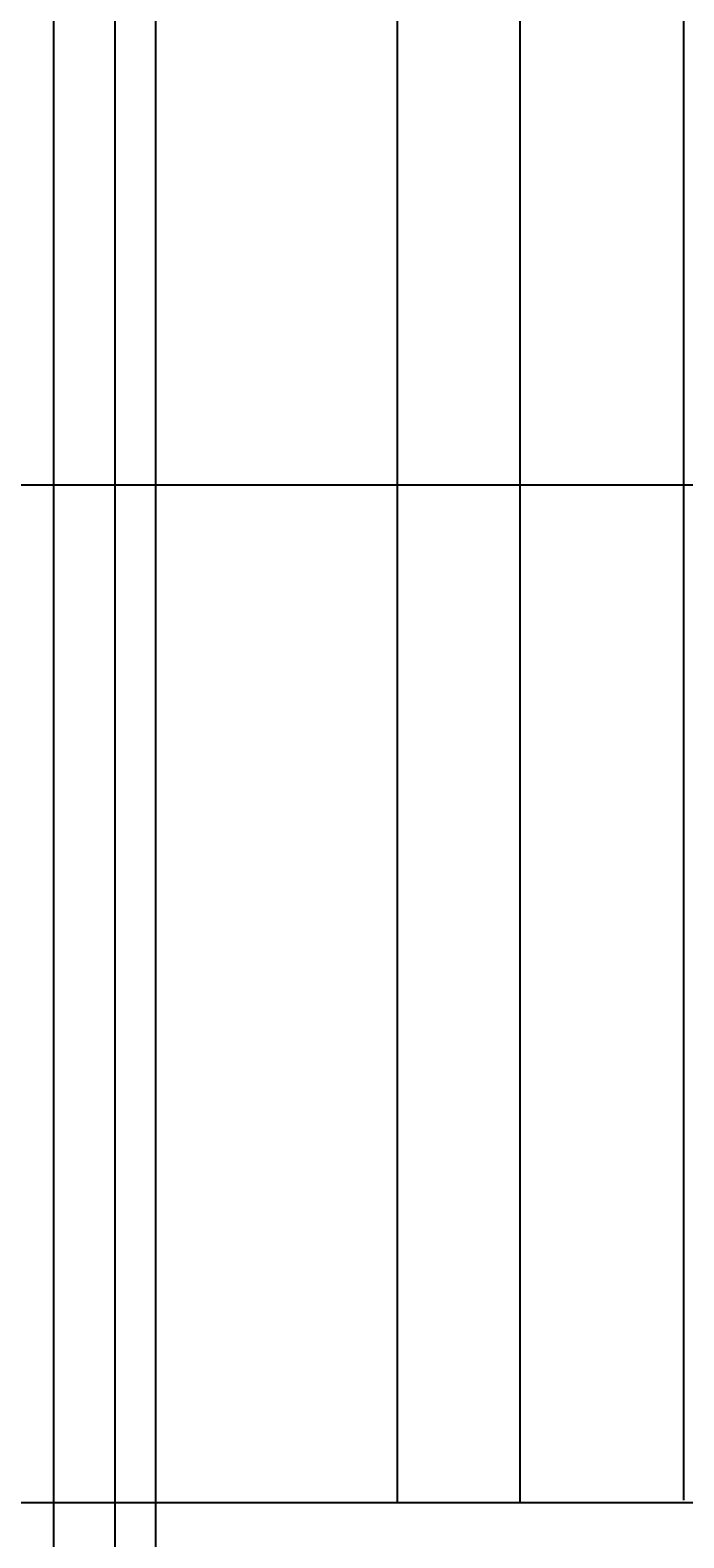
# Model space of a CAD drawing. Units: inches. Extents: x -6 to 289, y -8 to 323.
# Tile 21 of 107: x 126 to 142, y 50 to 87. Entities that reach past the tile are written whole.
import ezdxf

# ---------------------------------------------------------------- set-up
doc = ezdxf.new("R2010")
doc.units = ezdxf.units.IN
doc.header["$MEASUREMENT"] = 0
doc.layers.add('A-ANNO-DIMS', color=2, linetype='Continuous', lineweight=18)
doc.layers.add('A-DOOR', color=3, linetype='Continuous', lineweight=25)
doc.styles.get("Standard").update_dxf_attribs({"font": 'arial.ttf'})
doc.dimstyles.get("Standard").update_dxf_attribs({"dimtxt": 0.18, "dimasz": 0.18, "dimexe": 0.18, "dimexo": 0.0625, "dimgap": 0.09, "dimtad": 0, "dimtih": 1, "dimtoh": 1, "dimdec": 4, "dimzin": 0, "dimdsep": 46, "dimtxsty": 'Standard', "dimcen": 0.09, "dimadec": 0, "dimazin": 0, "dimtfac": 1, "dimtdec": 4, "dimtofl": 0, "dimtmove": 0, "dimatfit": 3, "dimfxl": 1, "dimtolj": 1, "dimtzin": 0, "dimarcsym": 0})

# ---------------------------------------------------------------- blocks, each defined once
blk = doc.blocks.new('*D16')
at = {"layer": 'A-ANNO-DIMS', "color": 0, "lineweight": -2, "transparency": 16777216}
for p, q in [((9.943, 68.37), (9.943, -8.391)), ((272.973, 68.37), (272.973, -8.391)), ((10.123, -8.211), (140.993, -8.211)), ((272.793, -8.211), (141.923, -8.211))]:
    blk.add_line(p, q, dxfattribs=at)
at = {"layer": 'A-ANNO-DIMS', "color": 0, "transparency": 16777216}
for points in [[(10.123, -8.181), (10.123, -8.241), (9.943, -8.211)], [(272.793, -8.181), (272.793, -8.241), (272.973, -8.211)]]:
    blk.add_solid(points, dxfattribs=at)
at = {"layer": 'Defpoints', "color": 0, "transparency": 16777216}
for p in [(9.943, 68.432), (272.973, 68.432), (272.973, -8.211)]:
    blk.add_point(p, dxfattribs=at)
at = {"layer": 'A-ANNO-DIMS', "color": 0, "transparency": 16777216, "insert": (141.458, -8.211), "char_height": 0.18, "attachment_point": 5}
blk.add_mtext('\\A1;263.03', dxfattribs=at)
blk = doc.blocks.new('*D28')
at = {"layer": 'A-ANNO-DIMS', "color": 0, "lineweight": -2, "transparency": 16777216}
for p, q in [((128.383, 180.092), (128.383, -8.391)), ((126.883, 178.592), (126.883, -8.391)), ((127.063, -8.211), (127.387, -8.211)), ((128.203, -8.211), (127.88, -8.211))]:
    blk.add_line(p, q, dxfattribs=at)
at = {"layer": 'A-ANNO-DIMS', "color": 0, "transparency": 16777216}
for points in [[(127.063, -8.181), (127.063, -8.241), (126.883, -8.211)], [(128.203, -8.181), (128.203, -8.241), (128.383, -8.211)]]:
    blk.add_solid(points, dxfattribs=at)
at = {"layer": 'Defpoints', "color": 0, "transparency": 16777216}
for p in [(128.383, 180.154), (126.883, 178.654), (128.383, -8.211)]:
    blk.add_point(p, dxfattribs=at)
at = {"layer": 'A-ANNO-DIMS', "color": 0, "transparency": 16777216, "insert": (127.633, -8.211), "char_height": 0.18, "attachment_point": 5}
blk.add_mtext('\\A1;1.5', dxfattribs=at)
blk = doc.blocks.new('*D29')
at = {"layer": 'A-ANNO-DIMS', "color": 0, "lineweight": -2, "transparency": 16777216}
for p, q in [((129.383, 181.092), (129.383, -8.391)), ((128.383, 180.092), (128.383, -8.391)), ((128.563, -8.211), (128.76, -8.211)), ((129.203, -8.211), (129.007, -8.211))]:
    blk.add_line(p, q, dxfattribs=at)
at = {"layer": 'A-ANNO-DIMS', "color": 0, "transparency": 16777216}
for points in [[(128.563, -8.181), (128.563, -8.241), (128.383, -8.211)], [(129.203, -8.181), (129.203, -8.241), (129.383, -8.211)]]:
    blk.add_solid(points, dxfattribs=at)
at = {"layer": 'Defpoints', "color": 0, "transparency": 16777216}
for p in [(129.383, 181.154), (128.383, 180.154), (129.383, -8.211)]:
    blk.add_point(p, dxfattribs=at)
at = {"layer": 'A-ANNO-DIMS', "color": 0, "transparency": 16777216, "insert": (128.883, -8.211), "char_height": 0.18, "attachment_point": 5}
blk.add_mtext('\\A1;1', dxfattribs=at)
blk = doc.blocks.new('*D30')
at = {"layer": 'A-ANNO-DIMS', "color": 0, "lineweight": -2, "transparency": 16777216}
for p, q in [((129.383, 181.092), (129.383, -8.391)), ((146.883, 181.092), (146.883, -8.391)), ((129.563, -8.211), (137.817, -8.211)), ((146.703, -8.211), (138.449, -8.211))]:
    blk.add_line(p, q, dxfattribs=at)
at = {"layer": 'A-ANNO-DIMS', "color": 0, "transparency": 16777216}
for points in [[(129.563, -8.181), (129.563, -8.241), (129.383, -8.211)], [(146.703, -8.181), (146.703, -8.241), (146.883, -8.211)]]:
    blk.add_solid(points, dxfattribs=at)
at = {"layer": 'Defpoints', "color": 0, "transparency": 16777216}
for p in [(129.383, 181.154), (146.883, 181.154), (146.883, -8.211)]:
    blk.add_point(p, dxfattribs=at)
at = {"layer": 'A-ANNO-DIMS', "color": 0, "transparency": 16777216, "insert": (138.133, -8.211), "char_height": 0.18, "attachment_point": 5}
blk.add_mtext('\\A1;17.5', dxfattribs=at)
blk = doc.blocks.new('*D73')
at = {"layer": 'A-ANNO-DIMS', "color": 0, "lineweight": -2, "transparency": 16777216}
for p, q in [((121.008, 51.148), (121.008, 322.969)), ((121.188, 322.789), (127.697, 322.789)), ((135.116, 322.789), (128.607, 322.789)), ((135.296, 51.148), (135.296, 322.969))]:
    blk.add_line(p, q, dxfattribs=at)
at = {"layer": 'A-ANNO-DIMS', "color": 0, "transparency": 16777216}
for points in [[(121.188, 322.819), (121.188, 322.759), (121.008, 322.789)], [(135.116, 322.819), (135.116, 322.759), (135.296, 322.789)]]:
    blk.add_solid(points, dxfattribs=at)
at = {"layer": 'Defpoints', "color": 0, "transparency": 16777216}
for p in [(135.296, 322.789), (121.008, 51.085), (135.296, 51.085)]:
    blk.add_point(p, dxfattribs=at)
at = {"layer": 'A-ANNO-DIMS', "color": 0, "transparency": 16777216, "insert": (128.152, 322.789), "char_height": 0.18, "attachment_point": 5}
blk.add_mtext('\\A1;14.288', dxfattribs=at)
blk = doc.blocks.new('*D74')
at = {"layer": 'A-ANNO-DIMS', "color": 0, "lineweight": -2, "transparency": 16777216}
for p, q in [((135.296, 51.148), (135.296, 322.969)), ((135.476, 322.789), (136.647, 322.789)), ((138.116, 322.789), (136.945, 322.789)), ((138.296, 51.148), (138.296, 322.969))]:
    blk.add_line(p, q, dxfattribs=at)
at = {"layer": 'A-ANNO-DIMS', "color": 0, "transparency": 16777216}
for points in [[(135.476, 322.819), (135.476, 322.759), (135.296, 322.789)], [(138.116, 322.819), (138.116, 322.759), (138.296, 322.789)]]:
    blk.add_solid(points, dxfattribs=at)
at = {"layer": 'Defpoints', "color": 0, "transparency": 16777216}
for p in [(138.296, 322.789), (135.296, 51.085), (138.296, 51.085)]:
    blk.add_point(p, dxfattribs=at)
at = {"layer": 'A-ANNO-DIMS', "color": 0, "transparency": 16777216, "insert": (136.796, 322.789), "char_height": 0.18, "attachment_point": 5}
blk.add_mtext('\\A1;3', dxfattribs=at)
blk = doc.blocks.new('*D75')
at = {"layer": 'A-ANNO-DIMS', "color": 0, "lineweight": -2, "transparency": 16777216}
for p, q in [((138.296, 51.148), (138.296, 322.969)), ((138.476, 322.789), (140.144, 322.789)), ((142.116, 322.789), (140.448, 322.789)), ((142.296, 51.148), (142.296, 322.969))]:
    blk.add_line(p, q, dxfattribs=at)
at = {"layer": 'A-ANNO-DIMS', "color": 0, "transparency": 16777216}
for points in [[(138.476, 322.819), (138.476, 322.759), (138.296, 322.789)], [(142.116, 322.819), (142.116, 322.759), (142.296, 322.789)]]:
    blk.add_solid(points, dxfattribs=at)
at = {"layer": 'Defpoints', "color": 0, "transparency": 16777216}
for p in [(142.296, 322.789), (138.296, 51.085), (142.296, 51.085)]:
    blk.add_point(p, dxfattribs=at)
at = {"layer": 'A-ANNO-DIMS', "color": 0, "transparency": 16777216, "insert": (140.296, 322.789), "char_height": 0.18, "attachment_point": 5}
blk.add_mtext('\\A1;4', dxfattribs=at)
blk = doc.blocks.new('*D76')
at = {"layer": 'A-ANNO-DIMS', "color": 0, "lineweight": -2, "transparency": 16777216}
for p, q in [((142.296, 51.148), (142.296, 322.969)), ((142.476, 322.789), (153.076, 322.789)), ((164.116, 322.789), (153.516, 322.789)), ((164.296, 51.148), (164.296, 322.969))]:
    blk.add_line(p, q, dxfattribs=at)
at = {"layer": 'A-ANNO-DIMS', "color": 0, "transparency": 16777216}
for points in [[(142.476, 322.819), (142.476, 322.759), (142.296, 322.789)], [(164.116, 322.819), (164.116, 322.759), (164.296, 322.789)]]:
    blk.add_solid(points, dxfattribs=at)
at = {"layer": 'Defpoints', "color": 0, "transparency": 16777216}
for p in [(164.296, 322.789), (142.296, 51.085), (164.296, 51.085)]:
    blk.add_point(p, dxfattribs=at)
at = {"layer": 'A-ANNO-DIMS', "color": 0, "transparency": 16777216, "insert": (153.296, 322.789), "char_height": 0.18, "attachment_point": 5}
blk.add_mtext('\\A1;22', dxfattribs=at)
blk = doc.blocks.new('*D86')
at = {"layer": 'A-ANNO-DIMS', "color": 0, "lineweight": -2, "transparency": 16777216}
for p, q in [((166.233, 75.971), (-5.737, 75.971)), ((-5.557, 75.791), (-5.557, 63.71)), ((-5.557, 51.265), (-5.557, 63.346)), ((120.945, 51.085), (-5.737, 51.085))]:
    blk.add_line(p, q, dxfattribs=at)
at = {"layer": 'A-ANNO-DIMS', "color": 0, "transparency": 16777216}
for points in [[(-5.587, 75.791), (-5.527, 75.791), (-5.557, 75.971)], [(-5.587, 51.265), (-5.527, 51.265), (-5.557, 51.085)]]:
    blk.add_solid(points, dxfattribs=at)
at = {"layer": 'Defpoints', "color": 0, "transparency": 16777216}
for p in [(-5.557, 75.971), (166.296, 75.971), (121.008, 51.085)]:
    blk.add_point(p, dxfattribs=at)
at = {"layer": 'A-ANNO-DIMS', "color": 0, "transparency": 16777216, "insert": (-5.557, 63.528), "char_height": 0.18, "attachment_point": 5}
blk.add_mtext('\\A1;24.886', dxfattribs=at)
blk = doc.blocks.new('*D87')
at = {"layer": 'A-ANNO-DIMS', "color": 0, "lineweight": -2, "transparency": 16777216}
for p, q in [((142.233, 108.948), (-5.737, 108.948)), ((-5.557, 108.768), (-5.557, 92.641)), ((-5.557, 76.151), (-5.557, 92.277)), ((166.233, 75.971), (-5.737, 75.971))]:
    blk.add_line(p, q, dxfattribs=at)
at = {"layer": 'A-ANNO-DIMS', "color": 0, "transparency": 16777216}
for points in [[(-5.587, 108.768), (-5.527, 108.768), (-5.557, 108.948)], [(-5.587, 76.151), (-5.527, 76.151), (-5.557, 75.971)]]:
    blk.add_solid(points, dxfattribs=at)
at = {"layer": 'Defpoints', "color": 0, "transparency": 16777216}
for p in [(-5.557, 108.948), (142.296, 108.948), (166.296, 75.971)]:
    blk.add_point(p, dxfattribs=at)
at = {"layer": 'A-ANNO-DIMS', "color": 0, "transparency": 16777216, "insert": (-5.557, 92.459), "char_height": 0.18, "attachment_point": 5}
blk.add_mtext('\\A1;32.98', dxfattribs=at)

msp = doc.modelspace()

# ---------------------------------------------------------------- linework, layer by layer
at = {"layer": 'A-DOOR'}
for points in [[(135.296, 51.0851), (135.296, 117.9706), (171.296, 117.9706), (171.296, 51.0851)], [(138.296, 51.0851), (138.296, 114.9477), (168.296, 114.9477), (168.296, 51.0851)]]:
    msp.add_lwpolyline(points, dxfattribs=at)
msp.add_lwpolyline([(121.008, 51.0851), (247.2408, 51.0851), (247.2408, 7.2888), (121.008, 7.2888)], close=True, dxfattribs=at)

# ---------------------------------------------------------------- dimensions: what is measured, and where the dimension line sits
at = {"layer": 'A-ANNO-DIMS'}
for base, p1, p2, override, picture, middle in [((135.296, 322.7888), (121.008, 51.0851), (135.296, 51.0851), {"dimdec": 3, "dimlfac": 1, "dimrnd": 0, "dimzin": 0, "dimdsep": 46, "dimlunit": 2}, '*D73', (128.152, 322.7888)), ((138.296, 322.7888), (135.296, 51.0851), (138.296, 51.0851), {"dimdec": 0, "dimlfac": 1, "dimrnd": 0, "dimzin": 0, "dimdsep": 46, "dimlunit": 2}, '*D74', (136.796, 322.7888)), ((142.296, 322.7888), (138.296, 51.0851), (142.296, 51.0851), {"dimdec": 0, "dimlfac": 1, "dimrnd": 0, "dimzin": 0, "dimdsep": 46, "dimlunit": 2}, '*D75', (140.296, 322.7888)), ((164.296, 322.7888), (142.296, 51.0851), (164.296, 51.0851), {"dimdec": 0, "dimlfac": 1, "dimrnd": 0, "dimzin": 0, "dimdsep": 46, "dimlunit": 2}, '*D76', (153.296, 322.7888)), ((129.3835, -8.2112), (128.3835, 180.154), (129.3835, 181.154), {"dimdec": 0, "dimlfac": 1, "dimrnd": 0, "dimzin": 0, "dimdsep": 46, "dimlunit": 2}, '*D29', (128.8835, -8.2112)), ((146.8835, -8.2112), (129.3835, 181.154), (146.8835, 181.154), {"dimdec": 1, "dimlfac": 1, "dimrnd": 0, "dimzin": 0, "dimdsep": 46, "dimlunit": 2}, '*D30', (138.1335, -8.2112)), ((128.3835, -8.2112), (126.8835, 178.654), (128.3835, 180.154), {"dimdec": 1, "dimlfac": 1, "dimrnd": 0, "dimzin": 0, "dimdsep": 46, "dimlunit": 2}, '*D28', (127.6335, -8.2112)), ((272.9733, -8.2112), (9.943, 68.4322), (272.9733, 68.4322), {"dimdec": 2, "dimlfac": 1, "dimrnd": 0, "dimzin": 0, "dimdsep": 46, "dimlunit": 2}, '*D16', (141.4581, -8.2112))]:
    dim = msp.add_linear_dim(base=base, p1=p1, p2=p2, dimstyle='Standard', override=override, dxfattribs=at)
    dim.commit()
    dim.dimension.update_dxf_attribs({"geometry": picture, "text_midpoint": middle})
for base, p1, p2, override, picture, middle in [((-5.557, 108.9477), (166.296, 75.9706), (142.296, 108.9477), {"dimdec": 2, "dimlfac": 1, "dimrnd": 0, "dimzin": 0, "dimdsep": 46, "dimlunit": 2}, '*D87', (-5.557, 92.4592)), ((-5.557, 75.97064), (121.00798, 51.08513), (166.29599, 75.97064), {"dimdec": 3, "dimlfac": 1, "dimrnd": 0, "dimzin": 0, "dimdsep": 46, "dimlunit": 2}, '*D86', (-5.557, 63.52788))]:
    dim = msp.add_linear_dim(base=base, p1=p1, p2=p2, angle=90, dimstyle='Standard', override=override, dxfattribs=at)
    dim.commit()
    dim.dimension.update_dxf_attribs({"geometry": picture, "text_midpoint": middle})

doc.saveas('drawing.dxf')
